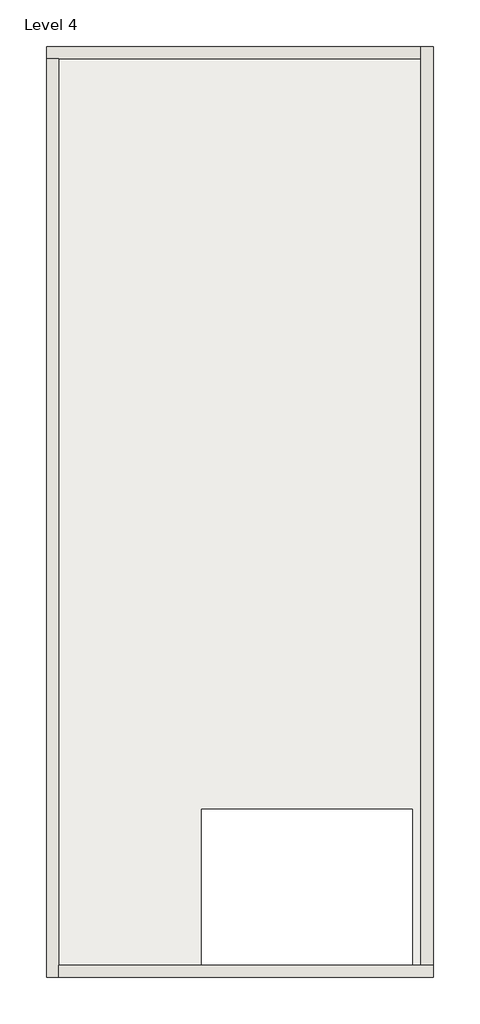
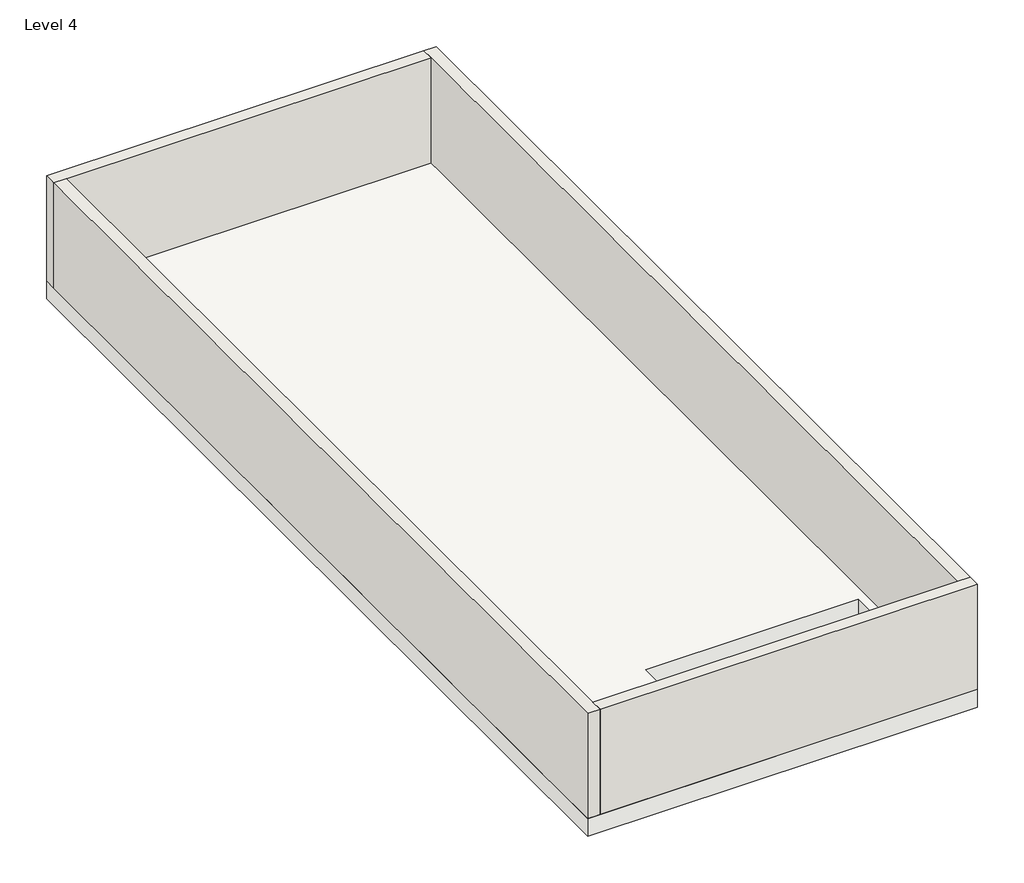
# One storey: 4 walls, 1 slab.
"""IFC4 building model written with IfcOpenShell, lengths in millimetres."""

from ifc_helpers import new_model, si_unit, frame, origin, place, context, project, spatial, polyline, outline, extrude, faceted_brep, element, save

model = new_model("IFC4")

# Units and contexts
model_context = context("Model", 3, world=origin())
ifc_project = project(units=[si_unit("LENGTHUNIT", "METRE", prefix="MILLI")], contexts=[model_context])

# Site, building, storey
site = spatial("IfcSite", under=ifc_project)
building = spatial("IfcBuilding", under=site)
storey = spatial("IfcBuildingStorey", under=building, Name="Level 4", Elevation=9601.2)

# Slab
placement = place(None, origin())
element("IfcSlab", 1, ObjectType="6\"", at=placement, inside=storey, context=model_context, shape_type="SweptSolid", body=[
    extrude(outline(polyline([(-3102.680937, 3065.0335625), (-3102.680937, -4631.1664375), (-6303.080937, -4631.1664375), (-6303.080937, 3065.0335625), (-3102.680937, 3065.0335625)]), holes=[polyline([(-5021.7909298, -3238.4779636), (-5021.7909298, -4554.9664375), (-3275.5409298, -4554.9664375), (-3275.5409298, -3238.4779636), (-5021.7909298, -3238.4779636)])]), frame((0.0, 0.0, 9448.8), z_axis=(0.0, 0.0, 1.0), x_axis=(1.0, 0.0, 0.0)), (0.0, 0.0, 1.0), 152.4),
])

# Walls
element("IfcWall", 2, ObjectType="4\"", at=placement, inside=storey, context=model_context, shape_type="Brep", body=[
    faceted_brep([(-6303.080937, 2963.4335625, 9601.2), (-6201.480937, 2963.4335625, 9601.2), (-3204.280937, 2963.4335625, 9601.2), (-3204.280937, 2963.4335625, 10515.6), (-6201.480937, 2963.4335625, 10515.6), (-6303.080937, 2963.4335625, 10515.6), (-6303.080937, 3065.0335625, 9601.2), (-6303.080937, 3065.0335625, 10515.6), (-3204.280937, 3065.0335625, 10515.6), (-3204.280937, 3065.0335625, 9601.2)], [[[0, 1, 2, 3, 4, 5]], [[6, 7, 8, 9]], [[2, 1, 0, 6, 9]], [[5, 4, 3, 8, 7]], [[0, 5, 7, 6]], [[3, 2, 9, 8]]]),
])
element("IfcWall", 3, ObjectType="4\"", at=placement, inside=storey, context=model_context, shape_type="Brep", body=[
    faceted_brep([(-6201.480937, -4631.1664375, 9601.2), (-6201.480937, -4529.5664375, 9601.2), (-6201.480937, 2963.4335625, 9601.2), (-6201.480937, 2963.4335625, 10515.6), (-6201.480937, -4529.5664375, 10515.6), (-6201.480937, -4631.1664375, 10515.6), (-6303.080937, -4631.1664375, 9601.2), (-6303.080937, -4631.1664375, 10515.6), (-6303.080937, 2963.4335625, 10515.6), (-6303.080937, 2963.4335625, 9601.2)], [[[0, 1, 2, 3, 4, 5]], [[6, 7, 8, 9]], [[2, 1, 0, 6, 9]], [[5, 4, 3, 8, 7]], [[0, 5, 7, 6]], [[3, 2, 9, 8]]]),
])
element("IfcWall", 4, ObjectType="4\"", at=placement, inside=storey, context=model_context, shape_type="Brep", body=[
    faceted_brep([(-3102.680937, -4529.5664375, 9601.2), (-3204.280937, -4529.5664375, 9601.2), (-6201.480937, -4529.5664375, 9601.2), (-6201.480937, -4529.5664375, 10515.6), (-3204.280937, -4529.5664375, 10515.6), (-3102.680937, -4529.5664375, 10515.6), (-3102.680937, -4631.1664375, 9601.2), (-3102.680937, -4631.1664375, 10515.6), (-6201.480937, -4631.1664375, 10515.6), (-6201.480937, -4631.1664375, 9601.2)], [[[0, 1, 2, 3, 4, 5]], [[6, 7, 8, 9]], [[2, 1, 0, 6, 9]], [[5, 4, 3, 8, 7]], [[0, 5, 7, 6]], [[3, 2, 9, 8]]]),
])
element("IfcWall", 5, ObjectType="4\"", at=placement, inside=storey, context=model_context, shape_type="Brep", body=[
    faceted_brep([(-3204.280937, 3065.0335625, 9601.2), (-3204.280937, 2963.4335625, 9601.2), (-3204.280937, -4529.5664375, 9601.2), (-3204.280937, -4529.5664375, 10515.6), (-3204.280937, 2963.4335625, 10515.6), (-3204.280937, 3065.0335625, 10515.6), (-3102.680937, 3065.0335625, 9601.2), (-3102.680937, 3065.0335625, 10515.6), (-3102.680937, -4529.5664375, 10515.6), (-3102.680937, -4529.5664375, 9601.2)], [[[0, 1, 2, 3, 4, 5]], [[6, 7, 8, 9]], [[2, 1, 0, 6, 9]], [[5, 4, 3, 8, 7]], [[0, 5, 7, 6]], [[3, 2, 9, 8]]]),
])

save(model, "model.ifc")

# Revit data of these elements
# Type "6\""
#   Assembly Code = "B1010"
#   Function = 0
#   Layers, outside or top first: 0' - 6" no material (function 1)
# Type "4\""
#   Assembly Code = "B2010"
#   Layers, outside or top first: 0' - 4" no material (function 1)
# Element 1 (IfcSlab, "6\"")
#   Height Offset From Level = 0' - 0"
#   Phase Created = New Construction
#   Materials on its faces: "Default Floor"
# Elements 2, 3, 4, 5 (IfcWall, "4\"")
#   Top Offset = 0' - 0"
#   Base Offset = 0' - 0"
#   Unconnected Height = 3' - 0"
#   wall height = 3' - 0"
#   Phase Created = New Construction
#   Base Constraint = Level 4
#   Materials on its faces: "Default Wall"
# Materials
#   "Default Floor": colour RGB 128 128 128, transparency 0
#   "Default Wall": colour RGB 128 128 128, transparency 0
